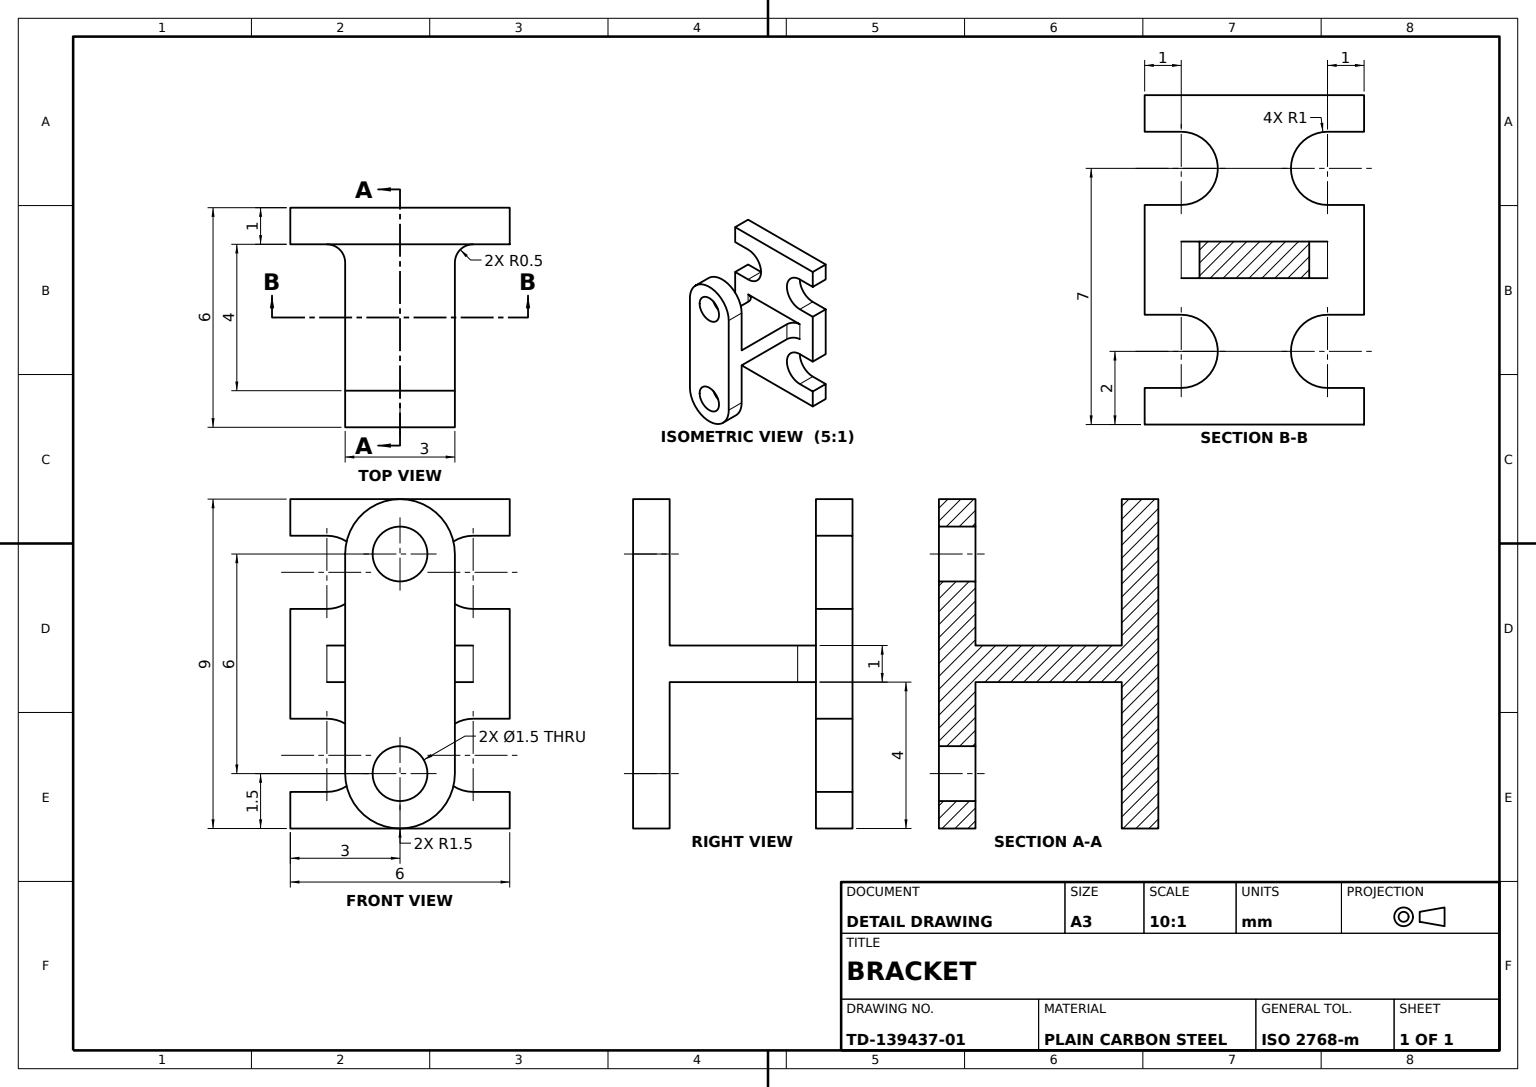
from build123d import *

# Parameters (mm, degrees)
BASE_PLATE_DEPTH         = 1
WEB_SKETCH_W             = 3
WEB_SKETCH_H             = 1
WEB_DEPTH                = 4
LINK_PLATE_SKETCH_R      = 0.75
LINK_PLATE_DEPTH         = 1
WEB_ROOT_FILLET_R0_5_A_R = 0.5
WEB_ROOT_FILLET_R0_5_B_R = 0.5


with BuildPart() as part:
    # Base Plate Sketch → Base Plate (new body)
    with BuildSketch(Plane.XY):
        with BuildLine():
            Line((-3, 3.5), (-2, 3.5))
            ThreePointArc((-2, 3.5), (-1, 2.5), (-2, 1.5))
            Line((-2, 1.5), (-3, 1.5))
            Line((-3, 1.5), (-3, -1.5))
            Line((-3, -1.5), (-2, -1.5))
            ThreePointArc((-2, -1.5), (-1, -2.5), (-2, -3.5))
            Line((-2, -3.5), (-3, -3.5))
            Line((-3, -3.5), (-3, -4.5))
            Line((-3, -4.5), (3, -4.5))
            Line((3, -4.5), (3, -3.5))
            Line((3, -3.5), (2, -3.5))
            ThreePointArc((2, -3.5), (1, -2.5), (2, -1.5))
            Line((2, -1.5), (3, -1.5))
            Line((3, -1.5), (3, 1.5))
            Line((3, 1.5), (2, 1.5))
            ThreePointArc((2, 1.5), (1, 2.5), (2, 3.5))
            Line((2, 3.5), (3, 3.5))
            Line((3, 3.5), (3, 4.5))
            Line((3, 4.5), (-3, 4.5))
            Line((-3, 4.5), (-3, 3.5))
        make_face()
    extrude(amount=BASE_PLATE_DEPTH)

    # Web Sketch → Web (add)
    with BuildSketch(Plane.XY.offset(1)):
        Rectangle(WEB_SKETCH_W, WEB_SKETCH_H)
    extrude(amount=WEB_DEPTH)

    # Link Plate Sketch → Link Plate (add)
    with BuildSketch(Plane.XY.offset(5)):
        with BuildLine():
            Line((1.5, 3), (1.5, -3))
            ThreePointArc((1.5, -3), (0, -4.5), (-1.5, -3))
            Line((-1.5, -3), (-1.5, 3))
            ThreePointArc((-1.5, 3), (0, 4.5), (1.5, 3))
        make_face()
        with Locations((0, 3)):
            Circle(LINK_PLATE_SKETCH_R, mode=Mode.SUBTRACT)
        with Locations((0, -3)):
            Circle(LINK_PLATE_SKETCH_R, mode=Mode.SUBTRACT)
    extrude(amount=LINK_PLATE_DEPTH)

    # Web Root Fillet R0.5 A
    web_root_fillet_r0_5_a_edges = [part.edges().sort_by_distance(p)[0] for p in [
        (1.5, 0, 1),
    ]]
    fillet(web_root_fillet_r0_5_a_edges, radius=WEB_ROOT_FILLET_R0_5_A_R)

    # Web Root Fillet R0.5 B
    web_root_fillet_r0_5_b_edges = [part.edges().sort_by_distance(p)[0] for p in [
        (-1.5, 0, 1),
    ]]
    fillet(web_root_fillet_r0_5_b_edges, radius=WEB_ROOT_FILLET_R0_5_B_R)


solid = part.part
